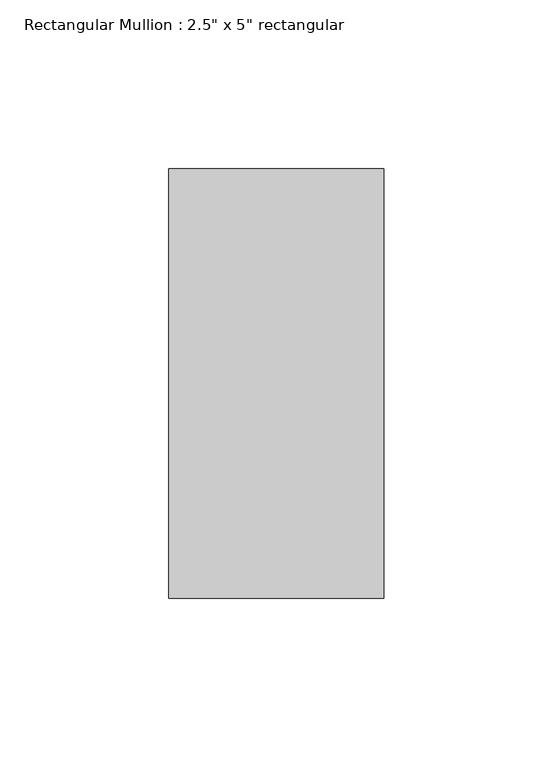
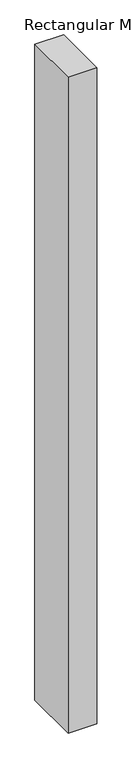
"""IFC4 building model written with IfcOpenShell, lengths in millimetres: member geometry."""

from ifc_helpers import new_model, si_unit, frame, origin, place, context, project, spatial, polyline, outline, extrude, source, transform, mapped, element, save


def member_8e1b9e66(model_context):
    return source(origin(), model_context, "Body", "SweptSolid", [
        extrude(outline(polyline([(0.0, 63.5), (0.0, -63.5), (-63.5, -63.5), (-63.5, 63.5), (0.0, 63.5)])), frame((0.0, 0.0, -1530.0793392), z_axis=(0.0, 0.0, 1.0), x_axis=(1.0, 0.0, 0.0)), (0.0, 0.0, 1.0), 1530.0793392),
    ])


if __name__ == "__main__":
    model = new_model("IFC4")
    model_context = context("Model", 3, world=origin())
    ifc_project = project(units=[si_unit("LENGTHUNIT", "METRE", prefix="MILLI")], contexts=[model_context])
    site = spatial("IfcSite", under=ifc_project)
    building = spatial("IfcBuilding", under=site)
    placement = place(None, origin())
    member_shape = member_8e1b9e66(model_context)
    element("IfcMember", 1, ObjectType="Rectangular Mullion : 2.5\" x 5\" rectangular", at=placement, inside=building, context=model_context, shape_type="MappedRepresentation", body=[
        mapped(member_shape, transform((0.0, 0.0, 0.0), x_axis=(1.0, 0.0, 0.0), y_axis=(0.0, 1.0, 0.0), z_axis=(0.0, 0.0, 1.0))),
    ])
    save(model, "model.ifc")

# Revit data of these elements
# Type "Rectangular Mullion : 2.5\" x 5\" rectangular"
#   built-in parameter 1007304 = 0.416667 (stored number, unit not read)
#   built-in parameter 1007301 = 0.104167 (stored number, unit not read)
#   built-in parameter 1007300 = 0.104167 (stored number, unit not read)
# Element 1 (IfcMember, "Rectangular Mullion : 2.5\" x 5\" rectangular")
#   Materials on its faces: "Aluminum"
# Materials
#   "Aluminum": class "Metal", colour RGB 247 247 247, transparency 0, Description = "Aluminum 6061", Cost = 0
